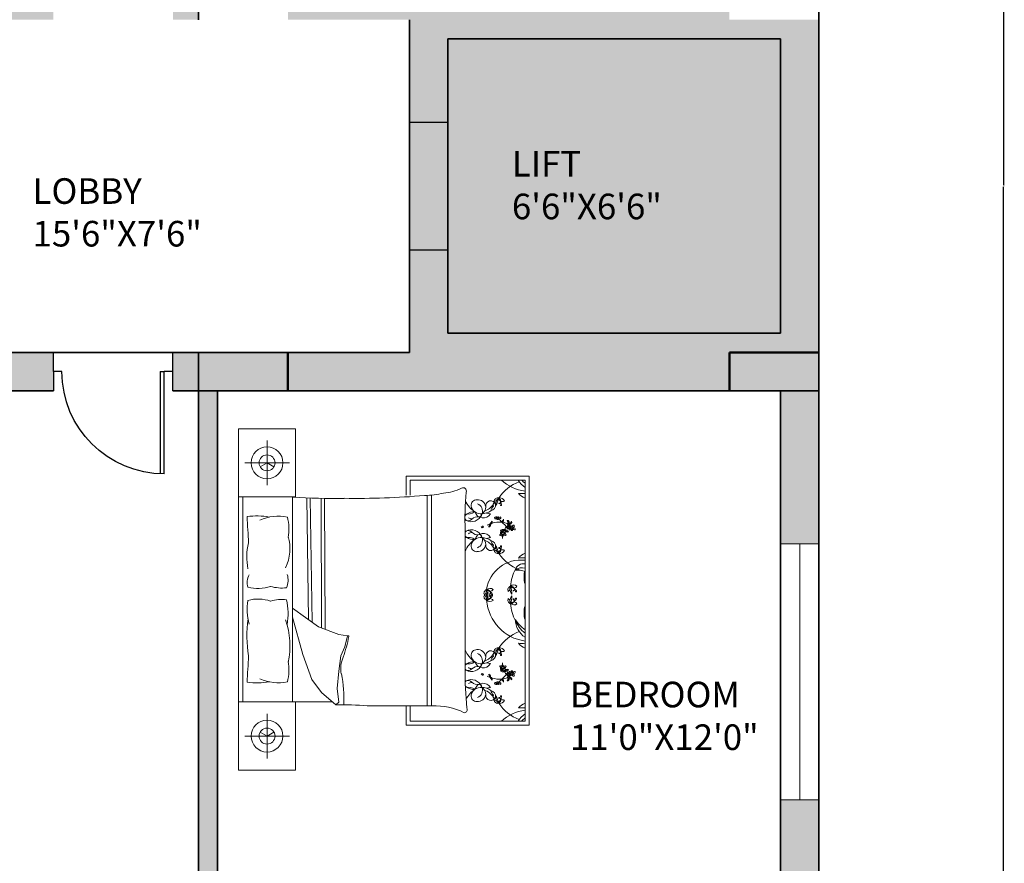
# Model space of a CAD drawing. Units: inches. Extents: x -28 to 485, y -861 to 54.
# Tile 5 of 14: x 254 to 485, y -563 to -365. Entities that reach past the tile are written whole.
import ezdxf

# ---------------------------------------------------------------- set-up
doc = ezdxf.new("R2010")
doc.units = ezdxf.units.IN
doc.header["$MEASUREMENT"] = 0
for name, color, linetype, lineweight in [('A-ANNO-DIMS', 2, 'Continuous', 18), ('A-AREA-IDEN', 7, 'Continuous', 18), ('A-COLS', 7, 'Continuous', 50), ('A-COLS-PATT', 8, 'Continuous', 13), ('A-DOOR', 3, 'Continuous', 25), ('A-DOOR-PATT', 9, 'Continuous', 13), ('A-FLOR-PATT', 42, 'Continuous', 13), ('A-FURN', 8, 'Continuous', 13), ('A-GLAZ', 4, 'Continuous', 18), ('A-WALL', 7, 'Continuous', 35), ('A-WALL-PATT', 34, 'Continuous', 13)]:
    doc.layers.add(name, color=color, linetype=linetype, lineweight=lineweight)
doc.styles.get("Standard").update_dxf_attribs({"font": 'arial.ttf'})
doc.dimstyles.get("Standard").update_dxf_attribs({"dimtxt": 0.18, "dimasz": 0.18, "dimexe": 0.18, "dimexo": 0.0625, "dimgap": 0.09, "dimtad": 0, "dimtih": 1, "dimtoh": 1, "dimdec": 0, "dimzin": 0, "dimdsep": 46, "dimlunit": 3, "dimtxsty": 'Standard', "dimcen": 0.09, "dimadec": 0, "dimazin": 0, "dimtfac": 1, "dimtdec": 0, "dimtofl": 0, "dimtmove": 0, "dimatfit": 3, "dimfxl": 1, "dimtolj": 1, "dimtzin": 0, "dimarcsym": 0})

# ---------------------------------------------------------------- blocks, each defined once
blk = doc.blocks.new('BED-DOUBLE-WITH-NIGHTSTANDS')
for p, q in [((0, 0), (0, 80.08)), ((6.67, 66.84), (6.67, 77.31)), ((11.91, 72.08), (1.44, 72.08)), ((39.26, 64.51), (39.26, 68.96)), ((39.26, 68.96), (68.11, 68.96)), ((40.19, 68.03), (40.19, 64.5)), ((67.18, 68.03), (40.19, 68.03)), ((67.18, 11.5), (67.18, 68.03)), ((68.11, 68.96), (68.11, 10.57)), ((1.03, 64.07), (1.03, 16.02)), ((12.66, 16.02), (12.66, 64.07)), ((15.98, 63.85), (16.38, 35.34)), ((16.8, 63.82), (17.22, 34.74)), ((19.33, 63.78), (19.45, 33.37)), ((20.15, 63.78), (20.27, 33.06)), ((44.25, 64.43), (44.25, 15.09)), ((45.25, 64.51), (45.25, 15.09)), ((59.06, 60.14), (58.15, 60.31)), ((53.12, 56.3), (53.12, 23.78)), ((59.06, 54.54), (58.15, 54.36)), ((12.66, 38.02), (18.76, 33.63)), ((15.04, 27.14), (12.66, 35.87)), ((18.76, 33.63), (23.47, 31.84)), ((23.47, 31.84), (25.57, 31.52)), ((25.57, 31.52), (24.92, 28.93)), ((24.92, 28.93), (23.95, 26.82)), ((17.14, 21.3), (15.04, 27.14)), ((23.95, 26.82), (23.47, 23.25)), ((23.47, 23.25), (23.14, 19.19)), ((59.06, 24.99), (58.15, 25.16)), ((19.41, 18.22), (17.14, 21.3)), ((23.14, 19.19), (23.47, 15.95)), ((59.06, 19.39), (58.15, 19.21)), ((22.82, 15.3), (19.41, 18.22)), ((0, 16.02), (21.98, 16.02)), ((23.47, 15.95), (22.82, 15.3)), ((39.26, 10.57), (39.26, 15.1)), ((40.19, 15.1), (40.19, 11.5)), ((6.67, 13.24), (6.67, 2.78)), ((68.11, 10.57), (39.26, 10.57)), ((40.19, 11.5), (67.18, 11.5)), ((11.91, 8.01), (1.44, 8.01))]:
    blk.add_line(p, q)
for points in [[(0, 64.07), (13.35, 64.07), (13.35, 80.08), (0, 80.08)], [(6.67, 72.08), (5.06, 71.14)], [(6.67, 72.08), (8.29, 71.14)], [(13.35, 16.02), (13.35, 0), (0, 0)], [(6.67, 8.01), (5.06, 8.94)], [(6.67, 8.01), (8.29, 8.94)]]:
    blk.add_lwpolyline(points)
for points in [[(43.62, 64.41, 0.056112), (48.03, 64.99, 0.095341), (52.27, 66.12)], [(2, 59.47, -0.074897), (7.23, 59.37, 0.472817)], [(7.52, 43.09, -0.14099), (2.18, 42.93, -0.235245)], [(7.52, 39.67, 0.14099), (2.18, 39.83, 0.235245)], [(2, 20.62, 0.074897), (7.23, 20.71, -0.472817)], [(30.15, 15.13, 0.001242), (45.35, 15.09, -0.127202), (52.92, 13.49)]]:
    blk.add_lwpolyline(points, format="xyb")
for centre, radius in [((6.67, 72.08), 3.74), ((6.67, 72.08), 1.87), ((61.96, 55.51), 0.204), ((64.11, 56.84), 0.204), ((61.96, 24.02), 0.204), ((64.11, 22.68), 0.204), ((6.67, 8.01), 3.74), ((6.67, 8.01), 1.87)]:
    blk.add_circle(centre, radius)
for centre, radius, start, end in [((69.62, 57.92), 10.46, 111.4092, 145.6135), ((68.59, 75.81), 10.46, 228.1144, 262.255), ((69.99, 70.57), 5.1, 209.8884, 236.5383), ((70.94, 72.4), 6.35, 223.5186, 233.6964), ((52.68, 65.51), 0.73, 336.5219, 123.8264), ((131.01, 58.75), 77.93, 175.2402, 181.8035), ((68.81, 67.71), 4.25, 221.0454, 247.4453), ((66.52, 79.36), 14.47, 266.3481, 272.5919), ((22.44, 207.63), 143.9, 266.1, 270.9282), ((27.68, 251.44), 187.71, 269.1145, 274.8735), ((58.76, 65.61), 6.06, 203.6453, 236.3329), ((55.85, 62.08), 1.35, 88.9462, 185.5144), ((56.04, 61.53), 1.91, 7.1143, 95.0551), ((55.32, 60.77), 1.86, 338.5779, 68.4181), ((56.48, 64.35), 3.78, 288.2955, 328.7386), ((59.12, 61.97), 1.2, 19.1312, 189.736), ((58.76, 62.26), 1.5, 285.6955, 4.031), ((60.43, 62.21), 0.737, 126.7319, 206.0245), ((60.79, 62.99), 0.867, 76.272, 177.0484), ((59.47, 64.76), 1.79, 284.7031, 328.6173), ((61.96, 62.49), 1.65, 125.7657, 194.5347), ((53.85, 65.41), 7.32, 332.8176, 347.4827), ((61.24, 62.69), 1.16, 20.9613, 102.2885), ((61.86, 63.85), 0.873, 181.7131, 301.5367), ((59, 62.09), 2.64, 2.0648, 41.1598), ((60.59, 63.07), 0.856, 316.2238, 62.3173), ((61.09, 62.57), 0.0682, 20.2667, 316.2271), ((54, 59.28), 0.964, 127.675, 162.5814), ((53.71, 63.39), 3.32, 259.249, 301.1782), ((55.15, 57.49), 3.09, 85.2696, 124.215), ((56.85, 62.5), 2.41, 193.079, 274.7067), ((57.33, 61.13), 1.99, 196.8663, 330.0915), ((55.15, 57.49), 3.09, 53.6555, 57.2989), ((55.62, 61.86), 2.33, 305.9599, 357.6409), ((56.78, 64.39), 4.3, 273.4924, 303.7117), ((60.76, 60.64), 1.6, 128.4175, 173.8338), ((61.51, 62.18), 0.13, 168.5166, 2.0648), ((61.45, 62.19), 0.0631, 52.0591, 168.5166), ((-760.15, 15.33), 763.42, 2.85022, 3.31479), ((9.33, 49.26), 10.32, 78.2417, 114.8684), ((1.06, 56.61), 10.73, 348.9631, 14.8961), ((54, 59.28), 0.964, 196.6343, 225.5483), ((54.57, 60.82), 2.55, 240.8249, 340.7178), ((53.81, 59.69), 1.2, 246.1646, 318.4347), ((55.03, 61.2), 2.3, 240.0851, 262.564), ((55.94, 57.8), 1.64, 74.8529, 138.4347), ((56.5, 59.87), 0.497, 254.8529, 12.6959), ((61.28, 51.56), 6.63, 110.1059, 116.9968), ((59.16, 57.79), 0.163, 112.5583, 214.2343), ((59.06, 58.08), 0.384, 265.7131, 351.6568), ((58.72, 58.29), 0.671, 297.3659, 329.344), ((58.21, 58.87), 1.29, 313.6929, 321.7899), ((59.64, 57.99), 0.42, 115.5379, 168.6744), ((58.21, 58.6), 1.27, 329.344, 349.7412), ((61.28, 51.56), 6.63, 86.1723, 106.4158), ((57.2, 58.31), 2.26, 352.8698, 1.6736), ((60.19, 59.12), 0.158, 125.0752, 284.7644), ((60.43, 59.18), 0.34, 127.3642, 168.4363), ((60.17, 59.45), 0.49, 277.4968, 341.2737), ((60.56, 59.22), 0.195, 88.1325, 178.8919), ((60.95, 59.02), 0.422, 136.3462, 189.6513), ((60.71, 58.98), 0.176, 189.6513, 312.3208), ((60.75, 59.46), 0.204, 183.2768, 356.7232), ((61.39, 59.1), 0.668, 164.2829, 186.9148), ((60.6, 59.09), 0.334, 312.3208, 40.2111), ((61.31, 59.47), 0.474, 201.6382, 274.947), ((60.68, 58.82), 0.619, 42.3896, 66.5724), ((66.93, 63.72), 7.6, 217.9541, 226.8459), ((61.13, 59.18), 0.337, 10.9597, 52.2379), ((61.33, 59.15), 0.156, 274.947, 37.5263), ((61.86, 58.27), 0.163, 112.5583, 214.2343), ((61.75, 58.56), 0.384, 265.7131, 351.6568), ((61.42, 58.77), 0.671, 297.3659, 329.344), ((61.45, 54.86), 3.33, 60.7959, 85.244), ((54.37, 50.07), 10.94, 37.8256, 47.7588), ((60.91, 59.35), 1.29, 313.6929, 321.7899), ((62.33, 58.47), 0.42, 115.5379, 168.6744), ((60.9, 59.07), 1.27, 329.344, 349.7412), ((59.89, 58.78), 2.26, 352.8698, 1.6736), ((63.07, 58.33), 0.228, 33.0979, 123.1364), ((58.05, 55.12), 5.96, 31.1156, 34.8118), ((62.74, 57.94), 0.617, 2.3172, 70.5201), ((63.25, 57.78), 0.178, 135.7354, 318.1297), ((62.95, 58.07), 0.236, 315.7354, 31.1156), ((63.38, 57.79), 0.178, 68.2452, 250.6395), ((62.97, 58), 0.531, 352.6008, 57.1845), ((64.87, 54.44), 3.55, 111.7087, 116.2181), ((63.48, 58.12), 0.531, 252.8042, 349.6943), ((63.53, 58.17), 0.236, 248.2452, 323.6254), ((63.33, 58.31), 0.617, 291.7087, 3.0299), ((58.93, 61.56), 5.96, 323.6254, 327.3216), ((63.81, 58.16), 0.228, 325.6077, 55.6462), ((54, 55.39), 0.964, 134.4517, 156.7144), ((54.57, 53.85), 2.55, 19.2822, 119.1751), ((53.81, 54.99), 1.2, 41.5653, 113.8354), ((55.03, 53.47), 2.3, 97.436, 119.9149), ((55.94, 56.87), 1.64, 221.5653, 285.1471), ((57.33, 53.55), 1.99, 29.9085, 163.1337), ((57.16, 57.12), 0.251, 169.5864, 349.5616), ((57.25, 57.11), 0.154, 349.5616, 167.2949), ((59.06, 57.02), 0.42, 129.5056, 182.6421), ((57.85, 58), 1.27, 308.4388, 328.836), ((57.63, 59.02), 2.26, 296.5064, 305.3102), ((57.61, 57.86), 1.29, 336.3901, 344.4871), ((59.01, 57.53), 0.163, 83.9457, 185.6216), ((58.36, 57.69), 0.671, 328.836, 0.8141), ((58.71, 57.49), 0.384, 306.5232, 32.4668), ((61.65, 55.23), 0.34, 93.635, 168.4363), ((61.66, 57.07), 0.93, 253.6301, 325.4631), ((61.92, 55.78), 0.658, 82.0748, 142.6895), ((61.85, 56.68), 0.675, 228.342, 274.9894), ((61.6, 55.76), 0.2, 138.2946, 276.2474), ((61.68, 55.73), 0.278, 358.5719, 143.8954), ((61.77, 55.27), 0.195, 88.1325, 178.8919), ((61.84, 55.95), 0.281, 208.8493, 269.9355), ((61.6, 55.89), 0.321, 274.2123, 318.1587), ((61.87, 56.57), 0.565, 273.8774, 357.1501), ((62.58, 55.56), 0.643, 121.9501, 165.2442), ((62.09, 56.97), 0.547, 262.0748, 308.2393), ((62.13, 55.81), 0.135, 262.868, 7.094), ((61.89, 54.87), 0.619, 42.3896, 66.5724), ((62.12, 55.92), 0.403, 278.5614, 22.5914), ((62.34, 55.23), 0.337, 10.9597, 118.7804), ((65.87, 54.52), 3.99, 156.1523, 156.9499), ((62.34, 55.94), 0.202, 44.3732, 121.9501), ((62.97, 56.41), 0.565, 181.4625, 249.4747), ((62.87, 56.86), 0.547, 215.1128, 261.2773), ((63.31, 56.83), 0.93, 197.889, 269.722), ((65.87, 54.52), 3.99, 130.182, 149.456), ((63.02, 56.51), 0.675, 248.3627, 295.0101), ((62.69, 55.67), 0.658, 20.6625, 81.2773), ((63.67, 56.79), 0.658, 139.3812, 199.9959), ((62.44, 57.27), 0.93, 310.9365, 22.7695), ((62.87, 57.22), 0.675, 285.6484, 332.2957), ((62.75, 57.57), 0.547, 319.3812, 5.5456), ((61.45, 54.86), 3.33, 47.5083, 55.9967), ((62.97, 57.17), 0.565, 331.1838, 51.6792), ((63.55, 56.5), 0.158, 125.0752, 284.7644), ((63.8, 56.56), 0.34, 93.635, 168.4363), ((63.75, 57.1), 0.2, 138.2946, 276.2474), ((63.53, 56.83), 0.49, 277.4968, 341.2737), ((63.83, 57.07), 0.278, 358.5719, 143.8954), ((63.92, 56.61), 0.195, 88.1325, 178.8919), ((63.99, 57.29), 0.281, 208.8493, 269.9355), ((63.75, 57.22), 0.321, 274.2123, 318.1587), ((64.31, 56.4), 0.422, 136.3462, 189.6513), ((64.07, 56.36), 0.176, 189.6513, 312.3208), ((64.75, 56.48), 0.668, 164.2829, 186.9148), ((64.73, 56.9), 0.643, 121.9501, 165.2442), ((63.96, 56.47), 0.334, 312.3208, 40.2111), ((64.67, 56.85), 0.474, 201.6382, 274.947), ((64.28, 57.14), 0.135, 262.868, 7.094), ((64.04, 56.2), 0.619, 42.3896, 66.5724), ((64.27, 57.26), 0.403, 278.5614, 22.5914), ((64.49, 56.56), 0.337, 10.9597, 118.7804), ((64.49, 57.27), 0.202, 44.3732, 121.9501), ((64.7, 56.53), 0.156, 274.947, 37.5263), ((16.01, 49.96), 14.08, 166.3427, 191.1841), ((1.85, 51.98), 10.19, 333.8761, 16.1746), ((54, 55.39), 0.964, 203.2856, 232.325), ((53.71, 51.28), 3.32, 58.8218, 100.2867), ((58.76, 49.06), 6.06, 123.6671, 158.5059), ((55.15, 57.18), 3.09, 235.785, 274.7304), ((56.85, 52.18), 2.41, 85.2933, 166.921), ((55.32, 53.9), 1.86, 291.5819, 21.4221), ((56.5, 54.81), 0.497, 347.3041, 105.1471), ((55.15, 57.18), 3.09, 302.7011, 306.3445), ((55.62, 52.81), 2.33, 2.3591, 54.0401), ((56.78, 50.29), 4.3, 56.2883, 86.5076), ((56.48, 50.32), 3.78, 31.2614, 71.7045), ((60.76, 54.03), 1.6, 186.1662, 231.5825), ((58.76, 52.42), 1.5, 355.969, 74.3045), ((61.4, 55.17), 0.158, 125.0752, 284.7644), ((61.38, 55.5), 0.49, 277.4968, 341.2737), ((62.16, 55.06), 0.422, 136.3462, 189.6513), ((61.92, 55.02), 0.176, 189.6513, 312.3208), ((65.87, 54.52), 3.99, 175.2415, 182.8929), ((62.6, 55.14), 0.668, 164.2829, 186.9148), ((61.81, 55.14), 0.334, 312.3208, 40.2111), ((62.52, 55.52), 0.474, 201.6382, 274.947), ((62.55, 55.2), 0.156, 274.947, 37.5263), ((55.85, 52.59), 1.35, 174.4856, 271.0538), ((56.04, 53.15), 1.91, 264.9449, 352.8857), ((59.12, 52.71), 1.2, 170.264, 340.8688), ((60.43, 52.46), 0.737, 153.9755, 233.2681), ((60.79, 51.69), 0.867, 182.9516, 283.728), ((59.47, 49.92), 1.79, 31.3827, 75.2969), ((61.96, 52.19), 1.65, 165.4653, 234.2343), ((53.85, 49.26), 7.32, 12.5173, 27.1824), ((59, 52.59), 2.64, 318.8402, 357.9352), ((60.59, 51.6), 0.856, 297.6827, 43.7762), ((61.86, 50.82), 0.873, 58.4633, 178.2869), ((61.24, 51.98), 1.16, 257.7115, 339.0387), ((69.62, 56.75), 10.46, 214.3865, 248.5908), ((61.13, 52.12), 0.113, 43.7762, 339.7183), ((61.51, 52.5), 0.13, 357.9352, 191.4834), ((61.45, 52.48), 0.0631, 191.4834, 307.9409), ((68.81, 46.96), 4.25, 112.5547, 138.9546), ((66.17, 41.19), 8.09, 82.8636, 171.8197), ((66.52, 35.31), 14.47, 87.4081, 93.6519), ((74.19, 42.33), 10.46, 152.5854, 175.5377), ((66.74, 46.53), 1.88, 76.3898, 169.0739), ((66.48, 45.12), 2.37, 72.8609, 131.9049), ((65.43, 42.24), 4.68, 68.117, 96.6195), ((72.68, 45.26), 5.75, 162.9798, 196.4569), ((5.99, 44.03), 3.96, 153.3437, 196.1026), ((7.37, 44.56), 4.25, 335.0183, 18.5407), ((10.2, 52.53), 9.81, 254.1707, 275.9871), ((58.4, 41.51), 0.867, 106.1963, 206.9726), ((56.38, 42.39), 1.79, 314.6273, 358.5415), ((59.67, 41.66), 1.65, 155.6899, 224.4589), ((59.67, 40.53), 1.65, 135.5411, 204.3101), ((58.94, 41.49), 1.16, 50.8855, 132.2127), ((58.91, 42.8), 0.873, 211.6373, 331.4609), ((58.2, 41.49), 0.856, 346.148, 92.2415), ((57.3, 39.84), 2.64, 31.989, 71.0841), ((51.18, 40.16), 7.32, 2.7418, 17.407), ((51.18, 42.04), 7.32, 342.593, 357.2582), ((64.01, 42.31), 0.867, 106.1963, 206.9726), ((61.98, 43.19), 1.79, 314.6273, 358.5415), ((65.27, 42.46), 1.65, 155.6899, 224.4589), ((64.54, 42.29), 1.16, 50.8855, 132.2127), ((64.51, 43.6), 0.873, 211.6373, 331.4609), ((63.8, 42.29), 0.856, 346.148, 92.2415), ((62.91, 40.64), 2.64, 31.989, 71.0841), ((56.78, 40.96), 7.32, 2.7418, 17.407), ((64.47, 42.1), 0.0682, 50.1909, 346.0209), ((64.98, 41.95), 0.0631, 81.9833, 198.4408), ((65.04, 41.98), 0.13, 198.4408, 31.989), ((75.64, 42.98), 8.5, 174.3643, 175.6213), ((81.47, 38.5), 15.2, 160.0972, 160.2783), ((16.3, 37.72), 14.27, 171.5249, 193.96), ((10.2, 30.23), 9.81, 84.0129, 105.8293), ((-2.51, 36.66), 14.12, 349.8617, 13.6238), ((58.4, 40.68), 0.867, 153.0274, 253.8037), ((56.38, 39.81), 1.79, 1.4585, 45.3727), ((57.3, 42.35), 2.64, 288.9159, 328.011), ((58.2, 40.71), 0.856, 267.7585, 13.852), ((58.91, 39.39), 0.873, 28.5391, 148.3627), ((58.94, 40.71), 1.16, 227.7873, 309.1145), ((68.59, 40.66), 10.46, 184.4623, 262.255), ((58.87, 41.3), 0.0682, 50.1909, 346.0209), ((58.92, 40.88), 0.113, 13.852, 309.9245), ((59.44, 41.17), 0.13, 198.4408, 31.989), ((59.37, 41.15), 0.0631, 81.9833, 198.4408), ((59.44, 41.02), 0.13, 328.011, 161.5592), ((59.37, 41.04), 0.0631, 161.5592, 278.0167), ((64.01, 39.88), 0.867, 153.0274, 253.8037), ((61.98, 39.01), 1.79, 1.4585, 45.3727), ((65.27, 39.73), 1.65, 135.5411, 204.3101), ((56.78, 41.24), 7.32, 342.593, 357.2582), ((62.91, 41.55), 2.64, 288.9159, 328.011), ((63.8, 39.91), 0.856, 267.7585, 13.852), ((64.51, 38.59), 0.873, 28.5391, 148.3627), ((64.52, 40.08), 0.113, 13.852, 309.9245), ((64.98, 40.24), 0.0631, 161.5592, 278.0167), ((65.04, 40.22), 0.13, 328.011, 161.5592), ((64.54, 39.91), 1.16, 227.7873, 309.1145), ((74.19, 39.86), 10.46, 184.4623, 207.4146), ((72.68, 36.94), 5.75, 163.5431, 197.0202), ((75.64, 39.22), 8.5, 184.3787, 185.6357), ((81.47, 43.7), 15.2, 199.7217, 199.9028), ((30.98, 31.59), 29.04, 172.2196, 189.497), ((-6.57, 29.12), 18.61, 348.0397, 19.2615), ((69.99, 35.42), 5.1, 181.272, 236.5383), ((72.72, 40.59), 9.45, 214.0123, 234.053), ((70.94, 37.25), 6.35, 197.8504, 233.6964), ((69.62, 22.77), 10.46, 111.4092, 145.6135), ((-4.69, 37.08), 31.06, 340.1194, 349.3383), ((25.64, 31.34), 0.193, 358.8623, 109.7536), ((58.76, 30.46), 6.06, 201.4941, 236.3329), ((55.85, 26.93), 1.35, 88.9462, 185.5144), ((56.04, 26.38), 1.91, 7.1143, 95.0551), ((59.12, 26.82), 1.2, 19.1312, 189.736), ((60.79, 27.84), 0.867, 76.272, 177.0484), ((59.47, 29.61), 1.79, 284.7031, 328.6173), ((61.96, 27.34), 1.65, 125.7657, 194.5347), ((53.85, 30.27), 7.32, 332.8176, 347.4827), ((61.24, 27.55), 1.16, 20.9613, 102.2885), ((60.59, 27.92), 0.856, 316.2238, 62.3173), ((59, 26.94), 2.64, 2.0648, 41.1598), ((61.86, 28.71), 0.873, 181.7131, 301.5367), ((66.52, 44.21), 14.47, 266.3481, 272.5919), ((68.81, 32.56), 4.25, 221.0454, 247.4453), ((-760.15, 64.76), 763.42, 356.68521, 357.14978), ((1.06, 23.47), 10.73, 345.1039, 11.0369), ((30.48, 23.89), 6.52, 156.2616, 191.3392), ((53.71, 28.24), 3.32, 259.7133, 301.1782), ((55.15, 22.34), 3.09, 85.2696, 124.215), ((56.85, 27.35), 2.41, 193.079, 274.7067), ((57.33, 25.98), 1.99, 196.8663, 330.0915), ((55.32, 25.63), 1.86, 338.5779, 68.4181), ((55.62, 26.71), 2.33, 305.9599, 357.6409), ((56.78, 29.24), 4.3, 273.4924, 303.7117), ((56.48, 29.2), 3.78, 288.2955, 328.7386), ((58.76, 27.11), 1.5, 285.6955, 4.031), ((60.76, 25.49), 1.6, 128.4175, 173.8338), ((60.43, 27.07), 0.737, 126.7319, 206.0245), ((61.09, 27.42), 0.0682, 20.2667, 316.2271), ((61.51, 27.03), 0.13, 168.5166, 2.0648), ((61.45, 27.04), 0.0631, 52.0591, 168.5166), ((136.48, 22.83), 83.37, 179.3433, 185.6887), ((54, 24.13), 0.964, 127.675, 156.7144), ((54, 24.13), 0.964, 203.229, 225.5483), ((54.57, 25.67), 2.55, 240.8249, 340.7178), ((53.81, 24.54), 1.2, 246.1646, 318.4347), ((55.03, 26.06), 2.3, 240.0851, 262.564), ((55.94, 22.65), 1.64, 74.8529, 138.4347), ((56.5, 24.72), 0.497, 254.8529, 12.6959), ((55.15, 22.34), 3.09, 53.6555, 57.2989), ((61.4, 24.36), 0.158, 75.2356, 234.9248), ((61.65, 24.3), 0.34, 191.5637, 266.365), ((61.6, 23.76), 0.2, 83.7526, 221.7054), ((61.85, 22.84), 0.675, 85.0106, 131.658), ((61.66, 22.46), 0.93, 34.5369, 106.3699), ((61.92, 23.75), 0.658, 217.3105, 277.9252), ((61.38, 24.03), 0.49, 18.7263, 82.5032), ((61.68, 23.79), 0.278, 216.1046, 1.4281), ((61.77, 24.25), 0.195, 181.1081, 271.8675), ((61.84, 23.57), 0.281, 90.0645, 151.1507), ((61.6, 23.64), 0.321, 41.8413, 85.7877), ((61.92, 24.5), 0.176, 47.6792, 170.3487), ((62.16, 24.46), 0.422, 170.3487, 223.6538), ((65.87, 25.01), 3.99, 177.1071, 184.7585), ((61.87, 22.95), 0.565, 2.8499, 86.1226), ((62.6, 24.38), 0.668, 173.0852, 195.7171), ((62.58, 23.96), 0.643, 194.7558, 238.0499), ((62.09, 22.55), 0.547, 51.7607, 97.9252), ((61.81, 24.39), 0.334, 319.7889, 47.6792), ((62.52, 24.01), 0.474, 85.053, 158.3618), ((62.13, 23.71), 0.135, 352.906, 97.132), ((61.89, 24.66), 0.619, 293.4276, 317.6104), ((62.34, 24.29), 0.337, 241.2196, 349.0403), ((62.12, 23.6), 0.403, 337.4086, 81.4386), ((65.87, 25.01), 3.99, 203.0501, 203.8477), ((62.34, 23.59), 0.202, 238.0499, 315.6268), ((62.97, 23.11), 0.565, 110.5253, 178.5375), ((63.31, 22.7), 0.93, 90.278, 162.111), ((62.87, 22.67), 0.547, 98.7227, 144.8872), ((62.55, 24.33), 0.156, 322.4737, 85.053), ((63.02, 23.01), 0.675, 64.9899, 111.6373), ((62.69, 23.86), 0.658, 278.7227, 339.3375), ((63.55, 23.03), 0.158, 75.2356, 234.9248), ((63.53, 22.69), 0.49, 18.7263, 82.5032), ((64.07, 23.17), 0.176, 47.6792, 170.3487), ((64.31, 23.13), 0.422, 170.3487, 223.6538), ((64.75, 23.05), 0.668, 173.0852, 195.7171), ((63.96, 23.05), 0.334, 319.7889, 47.6792), ((64.67, 22.68), 0.474, 85.053, 158.3618), ((64.7, 22.99), 0.156, 322.4737, 85.053), ((9.33, 30.82), 10.32, 245.1316, 281.7583), ((-5.54, 16.67), 30.23, 357.4519, 11.3392), ((54, 20.25), 0.964, 134.4517, 153.558), ((54.57, 18.71), 2.55, 19.2822, 119.1751), ((53.81, 19.84), 1.2, 41.5653, 113.8354), ((57.16, 22.4), 0.251, 10.4384, 190.4136), ((57.25, 22.42), 0.154, 192.7051, 10.4384), ((61.28, 27.97), 6.63, 243.0032, 249.8941), ((57.85, 21.53), 1.27, 31.164, 51.5612), ((59.06, 22.5), 0.42, 177.3579, 230.4944), ((57.63, 20.5), 2.26, 54.6898, 63.4936), ((57.61, 21.66), 1.29, 15.5129, 23.6099), ((59.01, 21.99), 0.163, 174.3784, 276.0543), ((58.71, 22.03), 0.384, 327.5332, 53.4768), ((58.36, 21.84), 0.671, 359.1859, 31.164), ((59.16, 21.74), 0.163, 145.7657, 247.4417), ((59.06, 21.45), 0.384, 8.3432, 94.2869), ((58.72, 21.23), 0.671, 30.656, 62.6341), ((58.21, 20.66), 1.29, 38.2101, 46.3071), ((59.64, 21.53), 0.42, 191.3256, 244.4621), ((58.21, 20.93), 1.27, 10.2588, 30.656), ((61.28, 27.97), 6.63, 253.5842, 273.8277), ((57.2, 21.22), 2.26, 358.3264, 7.1302), ((66.93, 15.8), 7.6, 133.1541, 142.0459), ((61.86, 21.26), 0.163, 145.7657, 247.4417), ((54.37, 29.45), 10.94, 312.2412, 322.1744), ((61.45, 24.67), 3.33, 274.756, 299.2041), ((61.75, 20.97), 0.384, 8.3432, 94.2869), ((61.42, 20.76), 0.671, 30.656, 62.6341), ((60.91, 20.18), 1.29, 38.2101, 46.3071), ((62.33, 21.06), 0.42, 191.3256, 244.4621), ((60.9, 20.45), 1.27, 10.2588, 30.656), ((59.89, 20.74), 2.26, 358.3264, 7.1302), ((65.87, 25.01), 3.99, 210.544, 229.818), ((62.74, 21.59), 0.617, 289.4799, 357.6828), ((58.05, 24.41), 5.96, 325.1882, 328.8844), ((63.07, 21.2), 0.228, 236.8636, 326.9021), ((63.67, 22.74), 0.658, 160.0041, 220.6188), ((62.44, 22.26), 0.93, 337.2305, 49.0635), ((62.87, 22.31), 0.675, 27.7043, 74.3516), ((63.25, 21.74), 0.178, 41.8703, 224.2646), ((62.95, 21.45), 0.236, 328.8844, 44.2646), ((62.75, 21.95), 0.547, 354.4544, 40.6188), ((63.38, 21.74), 0.178, 109.3605, 291.7548), ((62.97, 21.52), 0.531, 302.8155, 7.3992), ((64.87, 25.09), 3.55, 243.7819, 248.2913), ((61.45, 24.67), 3.33, 304.0033, 312.4917), ((62.97, 22.35), 0.565, 308.3208, 28.8162), ((63.48, 21.4), 0.531, 10.3057, 107.1958), ((63.53, 21.36), 0.236, 36.3746, 111.7548), ((63.8, 22.96), 0.34, 191.5637, 266.365), ((63.75, 22.43), 0.2, 83.7526, 221.7054), ((63.33, 21.21), 0.617, 356.9701, 68.2913), ((63.83, 22.46), 0.278, 216.1046, 1.4281), ((63.92, 22.92), 0.195, 181.1081, 271.8675), ((58.93, 17.96), 5.96, 32.6784, 36.3746), ((63.99, 22.24), 0.281, 90.0645, 151.1507), ((63.75, 22.31), 0.321, 41.8413, 85.7877), ((63.81, 21.37), 0.228, 304.3538, 34.3923), ((64.73, 22.63), 0.643, 194.7558, 238.0499), ((64.28, 22.38), 0.135, 352.906, 97.132), ((64.04, 23.32), 0.619, 293.4276, 317.6104), ((64.49, 22.96), 0.337, 241.2196, 349.0403), ((64.27, 22.27), 0.403, 337.4086, 81.4386), ((64.49, 22.25), 0.202, 238.0499, 315.6268), ((54, 20.25), 0.964, 210.0293, 232.325), ((53.71, 16.14), 3.32, 58.8218, 99.1554), ((58.76, 13.91), 6.06, 123.6671, 153.2997), ((55.15, 22.04), 3.09, 235.785, 274.7304), ((55.03, 18.32), 2.3, 97.436, 119.9149), ((56.85, 17.03), 2.41, 85.2933, 166.921), ((55.94, 21.72), 1.64, 221.5653, 285.1471), ((57.33, 18.4), 1.99, 29.9085, 163.1337), ((55.32, 18.75), 1.86, 291.5819, 21.4221), ((56.5, 19.66), 0.497, 347.3041, 105.1471), ((55.15, 22.04), 3.09, 302.7011, 306.3445), ((55.62, 17.67), 2.33, 2.3591, 54.0401), ((56.78, 15.14), 4.3, 56.2883, 86.5076), ((56.48, 15.18), 3.78, 31.2614, 71.7045), ((58.76, 17.27), 1.5, 355.969, 74.3045), ((60.76, 18.89), 1.6, 186.1662, 231.5825), ((60.19, 20.41), 0.158, 75.2356, 234.9248), ((60.43, 20.35), 0.34, 191.5637, 232.6358), ((60.17, 20.07), 0.49, 18.7263, 82.5032), ((60.56, 20.3), 0.195, 181.1081, 271.8675), ((60.71, 20.55), 0.176, 47.6792, 170.3487), ((60.95, 20.51), 0.422, 170.3487, 223.6538), ((60.75, 20.06), 0.204, 3.2768, 176.7232), ((61.39, 20.43), 0.668, 173.0852, 195.7171), ((60.6, 20.43), 0.334, 319.7889, 47.6792), ((61.31, 20.06), 0.474, 85.053, 158.3618), ((60.68, 20.7), 0.619, 293.4276, 317.6104), ((61.13, 20.34), 0.337, 307.7621, 349.0403), ((61.33, 20.37), 0.156, 322.4737, 85.053), ((55.85, 17.44), 1.35, 174.4856, 271.0538), ((56.04, 18), 1.91, 264.9449, 352.8857), ((59.12, 17.56), 1.2, 170.264, 340.8688), ((60.43, 17.31), 0.737, 153.9755, 233.2681), ((59.47, 14.77), 1.79, 31.3827, 75.2969), ((60.79, 16.54), 0.867, 182.9516, 283.728), ((61.96, 17.04), 1.65, 165.4653, 234.2343), ((53.85, 14.11), 7.32, 12.5173, 27.1824), ((59, 17.44), 2.64, 318.8402, 357.9352), ((60.59, 16.46), 0.856, 297.6827, 43.7762), ((61.86, 15.67), 0.873, 58.4633, 178.2869), ((61.24, 16.83), 1.16, 257.7115, 339.0387), ((61.13, 16.97), 0.113, 43.7762, 339.7183), ((61.51, 17.35), 0.13, 357.9352, 191.4834), ((61.45, 17.33), 0.0631, 191.4834, 307.9409), ((24.81, -58.13), 73.46, 85.8294, 91.553), ((52.87, 14.23), 0.739, 273.98, 27.3412), ((69.62, 21.6), 10.46, 214.3865, 248.5908), ((68.59, 3.71), 10.46, 97.745, 131.8856), ((68.81, 11.81), 4.25, 112.5547, 138.9546), ((66.52, 0.17), 14.47, 87.4081, 93.6519), ((69.99, 8.96), 5.1, 123.4617, 150.1116), ((70.94, 7.13), 6.35, 126.3036, 136.4814)]:
    blk.add_arc(centre, radius, start, end)
blk = doc.blocks.new('DOOR-ENTRY-LEAF')
for p, q in [((23, 0), (23, 24)), ((24, 24), (24, 0)), ((23, 0), (24, 0))]:
    blk.add_line(p, q)
blk.add_arc((24, 0), 24, 90, 180)
blk = doc.blocks.new('WINDOW-60IN')
for p, q in [((0, 60), (0, 0)), ((9, 60), (0, 60)), ((4.5, 60), (4.5, 0)), ((9, 0), (9, 60)), ((0, 0), (9, 0))]:
    blk.add_line(p, q)
blk = doc.blocks.new('*D53')
at = {"layer": 'A-ANNO-DIMS', "color": 0, "lineweight": -2, "transparency": 16777216}
for p, q in [((441.35, 10.13), (484.71, 10.13)), ((484.53, 9.95), (484.53, -403.68)), ((484.53, -817.69), (484.53, -404.05)), ((441.35, -817.87), (484.71, -817.87))]:
    blk.add_line(p, q, dxfattribs=at)
at = {"layer": 'A-ANNO-DIMS', "color": 0, "transparency": 16777216}
for points in [[(484.5, 9.95), (484.56, 9.95), (484.53, 10.13)], [(484.5, -817.69), (484.56, -817.69), (484.53, -817.87)]]:
    blk.add_solid(points, dxfattribs=at)
at = {"layer": 'Defpoints', "color": 0, "transparency": 16777216}
for p in [(441.28, 10.13), (441.28, -817.87), (484.53, -817.87)]:
    blk.add_point(p, dxfattribs=at)
at = {"layer": 'A-ANNO-DIMS', "color": 0, "transparency": 16777216, "insert": (484.53, -403.87), "char_height": 0.18, "attachment_point": 5}
blk.add_mtext('\\A1;828', dxfattribs=at)

msp = doc.modelspace()

# ---------------------------------------------------------------- hatches: boundary and pattern name
at = {"layer": 'A-COLS-PATT'}
h = msp.add_hatch(color=256, dxfattribs=at)
h.dxf.hatch_style = 1
h.paths.add_polyline_path([(441.285, -591.367), (420.285, -591.367), (420.285, -595.867), (420.285, -600.367), (441.285, -600.367)])
h.paths.add_polyline_path([(304.691, -588.367), (295.785, -588.367), (295.785, -600.367), (304.691, -600.367)])
h.paths.add_polyline_path([(160.785, -588.367), (151.785, -588.367), (151.785, -600.367), (160.785, -600.367)])
h.paths.add_polyline_path([(36.285, -591.367), (24.285, -591.367), (15.285, -591.367), (15.285, -600.367), (36.285, -600.367)])
h.paths.add_polyline_path([(36.285, -808.867), (15.285, -808.867), (15.285, -817.867), (36.285, -817.867)])
h.paths.add_polyline_path([(160.785, -808.867), (139.785, -808.867), (139.785, -817.867), (160.785, -817.867)])
h.paths.add_polyline_path([(316.785, -808.867), (295.785, -808.867), (295.785, -817.867), (316.785, -817.867)])
h.paths.add_polyline_path([(441.285, -808.867), (420.285, -808.867), (420.285, -817.867), (441.285, -817.867)])
h.paths.add_polyline_path([(36.285, -442.867), (15.285, -442.867), (15.285, -451.867), (36.285, -451.867)])
h.paths.add_polyline_path([(160.785, -442.867), (139.785, -442.867), (139.785, -451.867), (160.785, -451.867)])
h.paths.add_polyline_path([(316.785, -442.867), (295.785, -442.867), (295.785, -451.867), (316.785, -451.867)])
h.paths.add_polyline_path([(441.285, -442.867), (420.285, -442.867), (420.285, -451.867), (441.285, -451.867)])
at = {"layer": 'A-DOOR-PATT'}
h = msp.add_hatch(color=256, dxfattribs=at)
h.dxf.hatch_style = 1
h.paths.add_polyline_path([(354.285, -388.867), (345.285, -388.867), (345.285, -418.867), (354.285, -418.867)])
at = {"layer": 'A-FLOR-PATT'}
h = msp.add_hatch(color=256, dxfattribs=at)
h.dxf.hatch_style = 1
h.paths.add_polyline_path([(432.285, -369.367), (354.285, -369.367), (354.285, -438.367), (432.285, -438.367)])
h.paths.add_polyline_path([(367.165, -414.955), (403.853, -414.955), (403.853, -392.566), (367.165, -392.566)], flags=24)
at = {"layer": 'A-WALL-PATT'}
h = msp.add_hatch(color=256, dxfattribs=at)
h.dxf.hatch_style = 1
h.paths.add_polyline_path([(160.785, -808.867), (160.785, -817.867), (295.785, -817.867), (295.785, -808.867)])
h.paths.add_polyline_path([(316.785, -817.867), (323.776, -817.867), (323.776, -808.867), (316.785, -808.867)])
h.paths.add_polyline_path([(420.285, -817.867), (420.285, -808.867), (383.776, -808.867), (383.776, -817.867)])
h.paths.add_polyline_path([(432.285, -808.867), (441.285, -808.867), (441.285, -702.966), (432.285, -702.966), (432.285, -708.367), (397.785, -708.367), (397.785, -710.617), (397.785, -712.867), (432.285, -712.867)])
h.paths.add_polyline_path([(300.285, -712.867), (329.285, -712.867), (329.285, -710.617), (329.285, -708.367), (295.785, -708.367), (295.785, -808.867), (300.285, -808.867)])
h.paths.add_polyline_path([(160.785, -698.867), (158.535, -698.867), (156.285, -698.867), (156.285, -808.867), (160.785, -808.867)])
h.paths.add_polyline_path([(36.285, -808.867), (36.285, -817.867), (79.721, -817.867), (79.721, -808.867)])
h.paths.add_polyline_path([(15.285, -808.867), (24.285, -808.867), (24.285, -739.09), (15.285, -739.09)])
h.paths.add_polyline_path([(24.285, -640.781), (15.285, -640.781), (15.285, -679.09), (24.285, -679.09), (24.285, -664.867), (89.285, -664.867), (89.285, -662.617), (89.285, -660.367), (24.285, -660.367)])
h.paths.add_polyline_path([(15.285, -616.781), (24.285, -616.781), (24.285, -600.367), (15.285, -600.367)])
h.paths.add_polyline_path([(36.285, -595.867), (36.285, -600.367), (123.285, -600.367), (123.285, -660.367), (117.285, -660.367), (117.285, -664.867), (156.285, -664.867), (156.285, -670.867), (160.785, -670.867), (160.785, -660.367), (127.785, -660.367), (127.785, -600.367), (129.785, -600.367), (129.785, -598.117), (129.785, -595.867)])
h.paths.add_polyline_path([(367.785, -664.867), (363.285, -664.867), (363.285, -708.367), (357.285, -708.367), (357.285, -712.867), (369.785, -712.867), (369.785, -708.367), (367.785, -708.367)])
h.paths.add_polyline_path([(432.285, -664.867), (432.285, -666.966), (441.285, -666.966), (441.285, -642.367), (432.285, -642.367), (432.285, -660.367), (328.785, -660.367), (328.785, -664.867), (363.285, -664.867)])
h.paths.add_polyline_path([(333.285, -600.367), (420.285, -600.367), (420.285, -595.867), (326.785, -595.867), (326.785, -600.367), (328.785, -600.367), (328.785, -630.367), (331.035, -630.367), (333.285, -630.367)])
h.paths.add_polyline_path([(441.285, -600.367), (432.285, -600.367), (432.285, -618.367), (441.285, -618.367)])
h.paths.add_polyline_path([(432.285, -591.367), (441.285, -591.367), (441.285, -547.793), (432.285, -547.793)])
h.paths.add_polyline_path([(295.785, -588.367), (300.238, -588.367), (300.285, -583.867), (300.285, -451.867), (295.785, -451.867)])
h.paths.add_polyline_path([(420.285, -451.867), (420.285, -442.867), (316.785, -442.867), (316.785, -451.867)])
h.paths.add_polyline_path([(432.285, -487.793), (441.285, -487.793), (441.285, -451.867), (432.285, -451.867)])
h.paths.add_polyline_path([(432.285, -442.867), (441.285, -442.867), (441.285, -364.867), (432.285, -364.867)])
h.paths.add_polyline_path([(261.785, -451.867), (261.785, -447.367), (261.785, -444.758), (261.785, -442.867), (160.785, -442.867), (160.785, -451.867)])
h.paths.add_polyline_path([(139.785, -451.867), (139.785, -442.867), (36.285, -442.867), (36.285, -451.867)])
h.paths.add_polyline_path([(15.285, -491.617), (24.285, -491.617), (24.285, -451.867), (15.285, -451.867)])
h.paths.add_polyline_path([(24.285, -551.617), (15.285, -551.617), (15.285, -591.367), (24.285, -591.367)])
h.paths.add_polyline_path([(160.785, -451.867), (156.285, -451.867), (156.285, -588.367), (160.785, -588.367)])
h.paths.add_polyline_path([(139.785, -364.867), (139.785, -355.867), (36.285, -355.867), (36.285, -364.867)])
h.paths.add_polyline_path([(24.285, -364.867), (15.285, -364.867), (15.285, -373.867), (24.285, -373.867)])
h.paths.add_polyline_path([(15.285, -433.867), (15.285, -442.867), (24.285, -442.867), (24.285, -433.867)])
h.paths.add_polyline_path([(261.785, -364.867), (261.785, -360.367), (261.785, -355.867), (160.785, -355.867), (160.785, -364.867)])
h.paths.add_polyline_path([(295.785, -355.867), (289.785, -355.867), (289.785, -364.867), (295.785, -364.867)])
h.paths.add_polyline_path([(295.785, -355.867), (300.285, -355.867), (300.285, -259.867), (333.285, -259.867), (333.285, -257.617), (333.285, -255.367), (300.285, -255.367), (300.285, -207.367), (295.785, -207.367)])
h.paths.add_polyline_path([(420.285, -364.867), (420.285, -355.867), (316.785, -355.867), (316.785, -364.867)])
h.paths.add_polyline_path([(24.285, -311.192), (15.285, -311.192), (15.285, -355.867), (24.285, -355.867)])
h.paths.add_polyline_path([(24.285, -211.867), (54.144, -211.867), (54.144, -207.367), (24.285, -207.367), (24.285, -187.772), (15.285, -187.772), (15.285, -251.192), (24.285, -251.192)])
h.paths.add_polyline_path([(82.144, -207.367), (82.144, -209.617), (82.144, -211.867), (127.785, -211.867), (127.785, -147.367), (129.785, -147.367), (129.785, -145.117), (129.785, -142.867), (36.285, -142.867), (36.285, -147.367), (123.285, -147.367), (123.285, -207.367)])
h.paths.add_polyline_path([(160.785, -207.367), (156.285, -207.367), (156.285, -355.867), (160.785, -355.867)])
h.paths.add_polyline_path([(24.285, 1.133), (15.285, 1.133), (15.285, -54.408), (24.285, -54.408)])
h.paths.add_polyline_path([(36.285, 10.133), (36.285, 1.133), (70.235, 1.133), (70.235, 10.133)])
h.paths.add_polyline_path([(15.285, -138.367), (24.285, -138.367), (24.285, -114.408), (15.285, -114.408)])
h.paths.add_polyline_path([(24.285, -147.367), (15.285, -147.367), (15.285, -163.772), (24.285, -163.772)])
h.paths.add_polyline_path([(156.285, -130.867), (160.785, -130.867), (160.785, 1.133), (156.285, 1.133)])
h.paths.add_polyline_path([(130.235, 1.133), (139.785, 1.133), (139.785, 10.133), (130.235, 10.133)])
h.paths.add_polyline_path([(316.785, 10.133), (316.785, 1.133), (328.097, 1.133), (328.097, 10.133)])
h.paths.add_polyline_path([(300.285, 1.133), (295.785, 1.133), (295.785, -130.867), (300.285, -130.867)])
h.paths.add_polyline_path([(420.285, -147.367), (420.285, -142.867), (326.785, -142.867), (326.785, -145.117), (326.785, -147.367), (328.785, -147.367), (328.785, -177.367), (331.035, -177.367), (333.285, -177.367), (333.285, -147.367)])
h.paths.add_polyline_path([(333.285, -207.367), (333.285, -205.367), (328.785, -205.367), (328.785, -211.867), (363.285, -211.867), (363.285, -255.367), (361.285, -255.367), (361.285, -259.867), (369.785, -259.867), (369.785, -255.367), (367.785, -255.367), (367.785, -211.867), (432.285, -211.867), (432.285, -214.893), (441.285, -214.893), (441.285, -188.008), (432.285, -188.008), (432.285, -207.367)])
h.paths.add_polyline_path([(441.285, -250.893), (432.285, -250.893), (432.285, -255.367), (397.785, -255.367), (397.785, -257.617), (397.785, -259.867), (432.285, -259.867), (432.285, -355.867), (441.285, -355.867)])
h.paths.add_polyline_path([(432.285, -138.367), (441.285, -138.367), (441.285, -115.099), (432.285, -115.099)])
h.paths.add_polyline_path([(441.285, -147.367), (432.285, -147.367), (432.285, -164.008), (441.285, -164.008)])
h.paths.add_polyline_path([(420.285, 1.133), (420.285, 10.133), (388.097, 10.133), (388.097, 1.133)])
h.paths.add_polyline_path([(432.285, -55.099), (441.285, -55.099), (441.285, 1.133), (432.285, 1.133)])
h = msp.add_hatch(color=256, dxfattribs=at)
h.dxf.hatch_style = 1
h.paths.add_polyline_path([(441.285, -364.867), (420.285, -364.867), (420.285, -355.867), (316.785, -355.867), (316.785, -364.867), (345.285, -364.867), (345.285, -388.867), (354.285, -388.867), (354.285, -369.367), (432.285, -369.367), (432.285, -438.367), (354.285, -438.367), (354.285, -418.867), (345.285, -418.867), (345.285, -442.867), (316.785, -442.867), (316.785, -451.867), (420.285, -451.867), (420.285, -442.867), (441.285, -442.867)])
h = msp.add_hatch(color=256, dxfattribs=at)
h.dxf.hatch_style = 1
h.paths.add_polyline_path([(354.285, -364.867), (345.285, -364.867), (345.285, -388.867), (354.285, -388.867)])
h.paths.add_polyline_path([(354.285, -418.867), (345.285, -418.867), (345.285, -442.867), (354.285, -442.867)])
h.paths.add_polyline_path([(295.785, -442.867), (289.785, -442.867), (289.785, -451.867), (295.785, -451.867)])

# ---------------------------------------------------------------- linework, layer by layer
at = {"layer": 'A-COLS'}
for p, q in [((316.785, -451.867), (316.785, -442.867)), ((420.285, -442.867), (420.285, -451.867)), ((420.285, -442.867), (441.285, -442.867))]:
    msp.add_line(p, q, dxfattribs=at)
at = {"layer": 'A-DOOR'}
for p, q in [((345.285, -388.867), (354.285, -388.867)), ((354.285, -418.867), (345.285, -418.867)), ((261.785, -444.758), (261.785, -442.867)), ((289.785, -451.867), (289.785, -442.867)), ((261.785, -447.367), (261.785, -444.758)), ((261.785, -444.758), (261.785, -444.758)), ((263.785, -447.367), (261.785, -447.367)), ((261.785, -447.367), (261.785, -451.867)), ((289.785, -447.367), (287.785, -447.367))]:
    msp.add_line(p, q, dxfattribs=at)
at = {"layer": 'A-WALL'}
for p, q in [((295.785, 10.133), (295.785, -364.867)), ((441.285, 10.133), (441.285, -817.867)), ((345.285, -364.867), (345.285, -442.867)), ((354.285, -369.367), (354.285, -438.367)), ((354.285, -369.367), (432.285, -369.367)), ((432.285, -369.367), (432.285, -438.367)), ((432.285, -438.367), (354.285, -438.367)), ((15.285, -442.867), (345.285, -442.867)), ((295.785, -442.867), (295.785, -817.867)), ((15.285, -451.867), (261.785, -451.867)), ((289.785, -451.867), (441.285, -451.867)), ((300.285, -451.867), (300.285, -583.867)), ((432.285, -451.867), (432.285, -591.367))]:
    msp.add_line(p, q, dxfattribs=at)

# ---------------------------------------------------------------- block references
at = {"layer": 'A-DOOR', "extrusion": (0, 0, -1), "zscale": -1, "rotation": 180}
msp.add_blockref('DOOR-ENTRY-LEAF', (-263.785, -447.367), dxfattribs=at)
at = {"layer": 'A-FURN'}
msp.add_blockref('BED-DOUBLE-WITH-NIGHTSTANDS', (305.203, -540.845), dxfattribs=at)
at = {"layer": 'A-GLAZ'}
msp.add_blockref('WINDOW-60IN', (432.285, -547.792), dxfattribs=at)

# ---------------------------------------------------------------- texts
at = {"layer": 'A-AREA-IDEN', "insert": (369.279, -395.654), "char_height": 6, "attachment_point": 1}
msp.add_mtext('LIFT\\P6\'6"X6\'6"', dxfattribs=at)
at = {"layer": 'A-AREA-IDEN', "char_height": 6, "attachment_point": 1}
for s, width, insert in [('LOBBY\\P15\'6"X7\'6"', 0.71873, (256.881, -402.044)), ('BEDROOM\\P11\'0"X12\'0"', 3.57677, (382.89, -520.095))]:
    msp.add_mtext_dynamic_manual_height_columns(s, width=width, gutter_width=1, heights=[0], dxfattribs=dict(at, insert=insert))

# ---------------------------------------------------------------- dimensions: what is measured, and where the dimension line sits
at = {"layer": 'A-ANNO-DIMS'}
dim = msp.add_linear_dim(base=(484.535, -817.867), p1=(441.285, 10.133), p2=(441.285, -817.867), angle=90, dimstyle='Standard', override={"dimdec": 0, "dimlfac": 1, "dimrnd": 0, "dimzin": 0, "dimdsep": 46, "dimlunit": 2}, dxfattribs=at)
dim.commit()
dim.dimension.update_dxf_attribs({"geometry": '*D53', "text_midpoint": (484.535, -403.867)})

doc.saveas('drawing.dxf')
